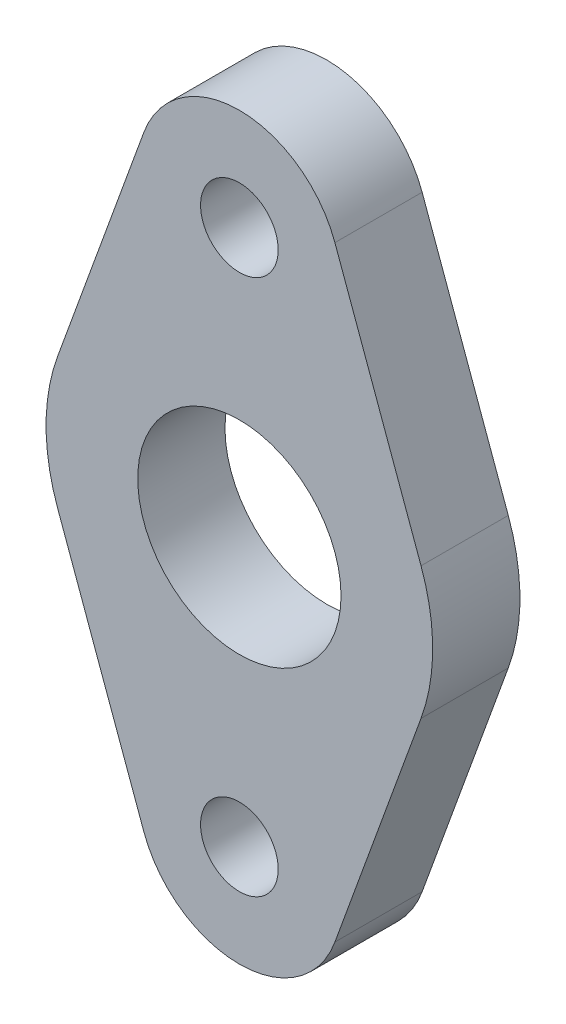
from build123d import *

# Parameters (mm, degrees)
FLANGE_PLATE_10_9MM_DEPTH             = 10.9
BORE_AND_BOLT_HOLES_SKETCH_R          = 4.85
BORE_AND_BOLT_HOLES_SKETCH_R_2        = 12.7
BORE_25_4_AND_BOLT_HOLES_2X_9_7_DEPTH = 49.9


with BuildPart() as part:
    # Flange Outline Sketch → Flange Plate 10.9mm (new body)
    with BuildSketch(Plane.XY):
        with BuildLine():
            Line((-11.935154873, 37.840746269), (-22.695589777, 8.254253731))
            ThreePointArc((-22.695589777, 8.254253731), (-24.15, 0), (-22.695589777, -8.254253731))
            Line((-22.695589777, -8.254253731), (-11.935154873, -37.840746269))
            ThreePointArc((-11.935154873, -37.840746269), (0, -46.2), (11.935154873, -37.840746269))
            Line((11.935154873, -37.840746269), (22.695589777, -8.254253731))
            ThreePointArc((22.695589777, -8.254253731), (24.15, 0), (22.695589777, 8.254253731))
            Line((22.695589777, 8.254253731), (11.935154873, 37.840746269))
            ThreePointArc((11.935154873, 37.840746269), (0, 46.2), (-11.935154873, 37.840746269))
        make_face()
    extrude(amount=FLANGE_PLATE_10_9MM_DEPTH)

    # Bore and Bolt Holes Sketch → Bore Ø25.4 and Bolt Holes 2xØ9.7 (cut)
    with BuildSketch(Plane.XY.offset(10.9)):
        with Locations((0, 33.5)):
            Circle(BORE_AND_BOLT_HOLES_SKETCH_R)
        with Locations((0, -33.5)):
            Circle(BORE_AND_BOLT_HOLES_SKETCH_R)
        Circle(BORE_AND_BOLT_HOLES_SKETCH_R_2)
    extrude(amount=-BORE_25_4_AND_BOLT_HOLES_2X_9_7_DEPTH, mode=Mode.SUBTRACT)


solid = part.part
